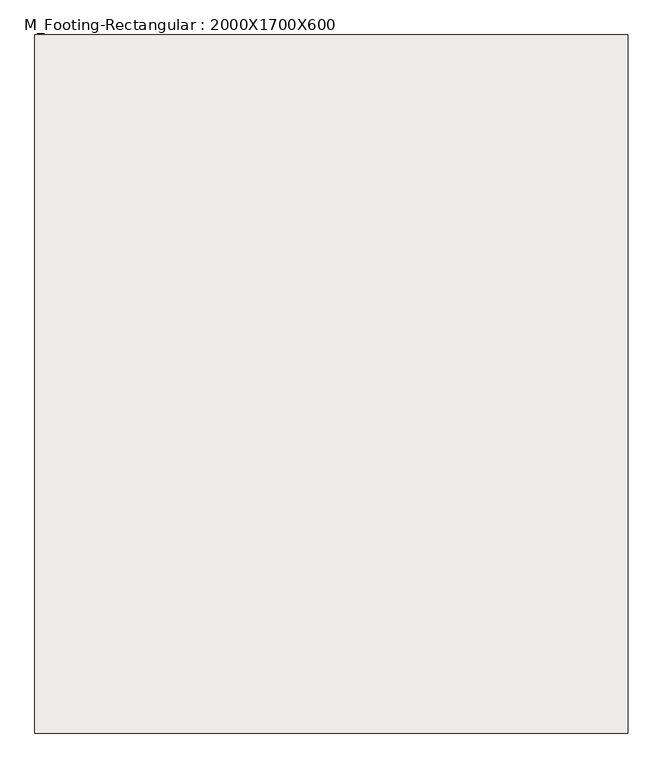
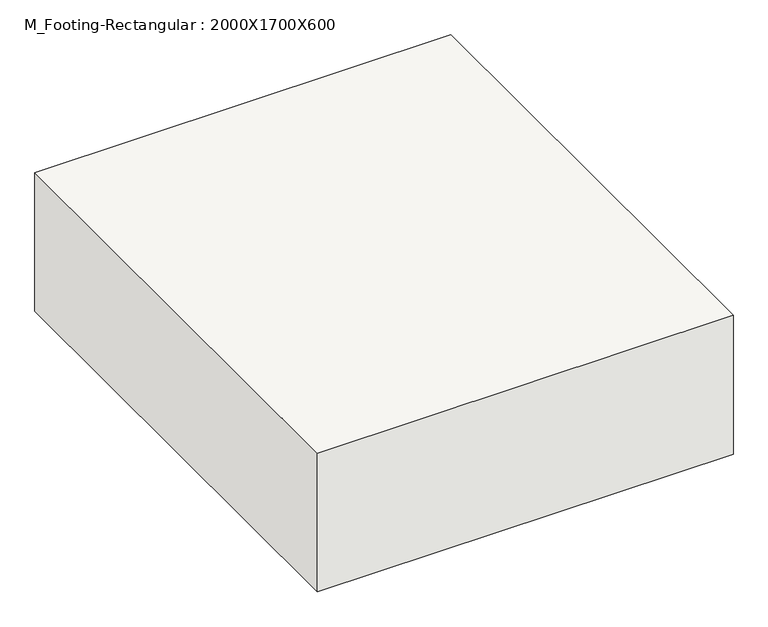
"""IFC4 building model written with IfcOpenShell, lengths in millimetres: slab geometry, M_Footing-Rectangular : 2000X1700X600."""

from ifc_helpers import new_model, si_unit, frame, origin, place, context, project, spatial, polyline, outline, extrude, source, transform, mapped, element, save


def m_footing_rectangular_2000x1700x600_e7f9a9ee(model_context):
    return source(origin(), model_context, "Body", "SweptSolid", [
        extrude(outline(polyline([(850.0, 1000.0), (850.0, -1000.0), (-850.0, -1000.0), (-850.0, 1000.0), (850.0, 1000.0)])), frame((0.0, 0.0, -600.0), z_axis=(0.0, 0.0, 1.0), x_axis=(1.0, 0.0, 0.0)), (0.0, 0.0, 1.0), 600.0),
    ])


if __name__ == "__main__":
    model = new_model("IFC4")
    model_context = context("Model", 3, world=origin())
    ifc_project = project(units=[si_unit("LENGTHUNIT", "METRE", prefix="MILLI")], contexts=[model_context])
    site = spatial("IfcSite", under=ifc_project)
    building = spatial("IfcBuilding", under=site)
    placement = place(None, origin())
    m_footing_rectangular_2000x1700x600_shape = m_footing_rectangular_2000x1700x600_e7f9a9ee(model_context)
    element("IfcSlab", 1, ObjectType="M_Footing-Rectangular : 2000X1700X600", at=placement, inside=building, context=model_context, shape_type="MappedRepresentation", body=[
        mapped(m_footing_rectangular_2000x1700x600_shape, transform((0.0, 0.0, 0.0), x_axis=(1.0, 0.0, 0.0), y_axis=(0.0, 1.0, 0.0), z_axis=(0.0, 0.0, 1.0))),
    ])
    save(model, "model.ifc")

# Revit data of these elements
# Type "M_Footing-Rectangular : 2000X1700X600"
#   Width = 1700 mm
#   Length = 2000 mm
#   Foundation Thickness = 600 mm
#   Structural Material [instance default] = Concrete, Cast-in-Place gray
#   Assembly Code = ""
# Element 1 (IfcSlab, "M_Footing-Rectangular : 2000X1700X600")
#   Structural Material = Concrete, Cast In Situ
#   Materials on its faces: "Concrete, Cast In Situ"
# Materials
#   "Concrete, Cast-in-Place gray": class "Concrete", colour RGB 192 192 192, transparency 0, Description = "Cast-in-place concrete", Cost = 0
#   "Concrete, Cast In Situ": class "Concrete", colour RGB 192 192 192, transparency 0, Description = "physical material", Cost = 0
